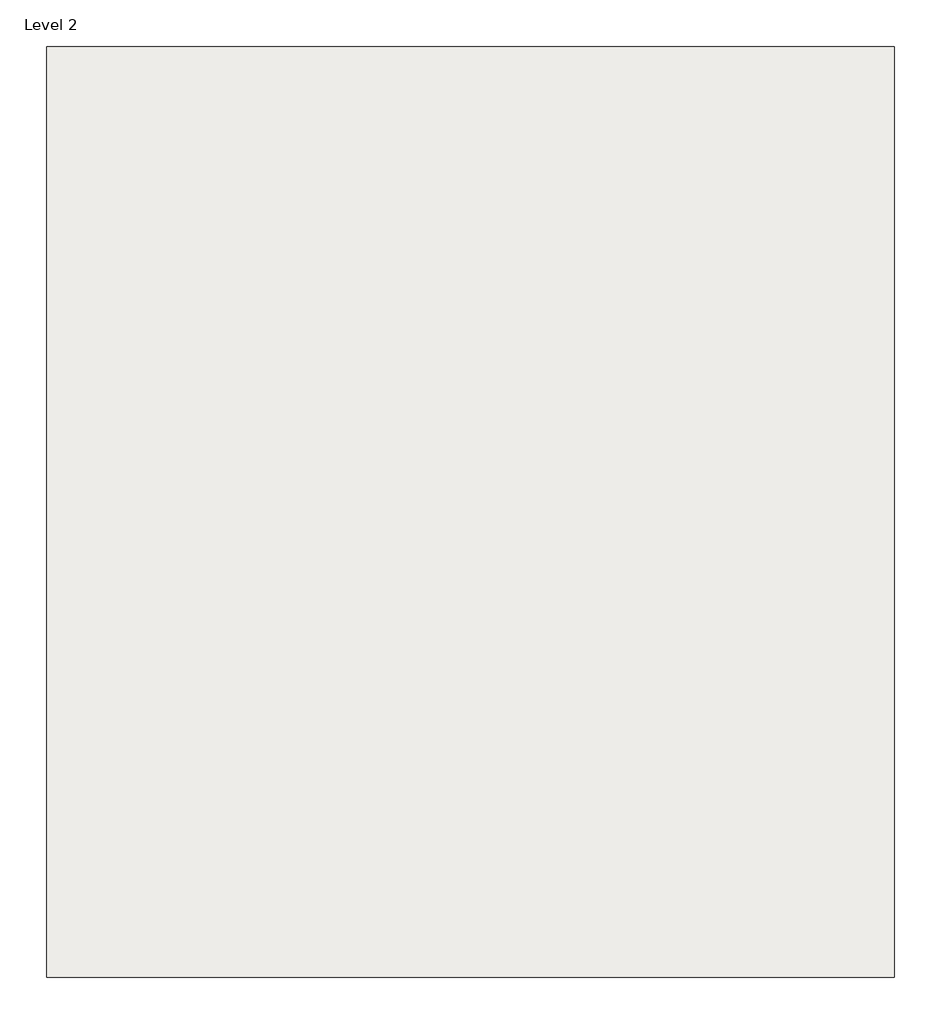
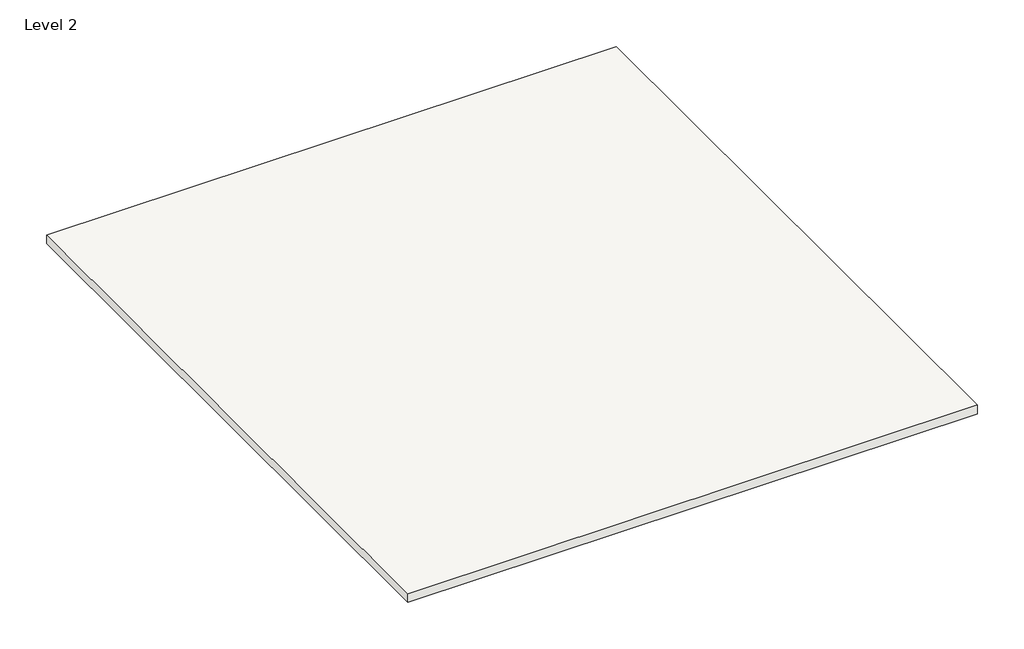
# One storey, incomplete: 1 roof.
"""IFC4 building model written with IfcOpenShell, lengths in millimetres."""

from ifc_helpers import new_model, si_unit, frame, origin, place, context, project, spatial, polyline, outline, extrude, element, save

model = new_model("IFC4")

# Units and contexts
model_context = context("Model", 3, world=origin())
ifc_project = project(units=[si_unit("LENGTHUNIT", "METRE", prefix="MILLI")], contexts=[model_context])

# Site, building, storey
site = spatial("IfcSite", under=ifc_project)
building = spatial("IfcBuilding", under=site)
storey = spatial("IfcBuildingStorey", under=building, Name="Level 2", Elevation=3048.0)

# Roof
placement = place(None, origin())
element("IfcRoof", 1, ObjectType="Generic - 12\"", at=placement, inside=storey, context=model_context, shape_type="SweptSolid", body=[
    extrude(outline(polyline([(-5539.1148498, 5385.7183073), (3909.6851502, 5385.7183073), (3909.6851502, -4993.3566927), (-5539.1148498, -4993.3566927), (-5539.1148498, 5385.7183073)])), frame((0.0, 0.0, 3048.0), z_axis=(0.0, 0.0, 1.0), x_axis=(1.0, 0.0, 0.0)), (0.0, 0.0, 1.0), 152.4),
])

save(model, "model.ifc")

# Revit data of these elements
# Type "Generic - 12\""
#   Assembly Code = "B1020"
#   Layers, outside or top first: 0' - 6" no material (function 1)
# Element 1 (IfcRoof, "Generic - 12\"")
#   built-in parameter 1001705 = 10.5 (stored number, unit not read)
#   built-in parameter 1001710 = 33615
#   Phase Created = New Construction
#   Materials on its faces: "Default Roof"
# Materials
#   "Default Roof": colour RGB 88 101 114, transparency 0, Cost = 0
